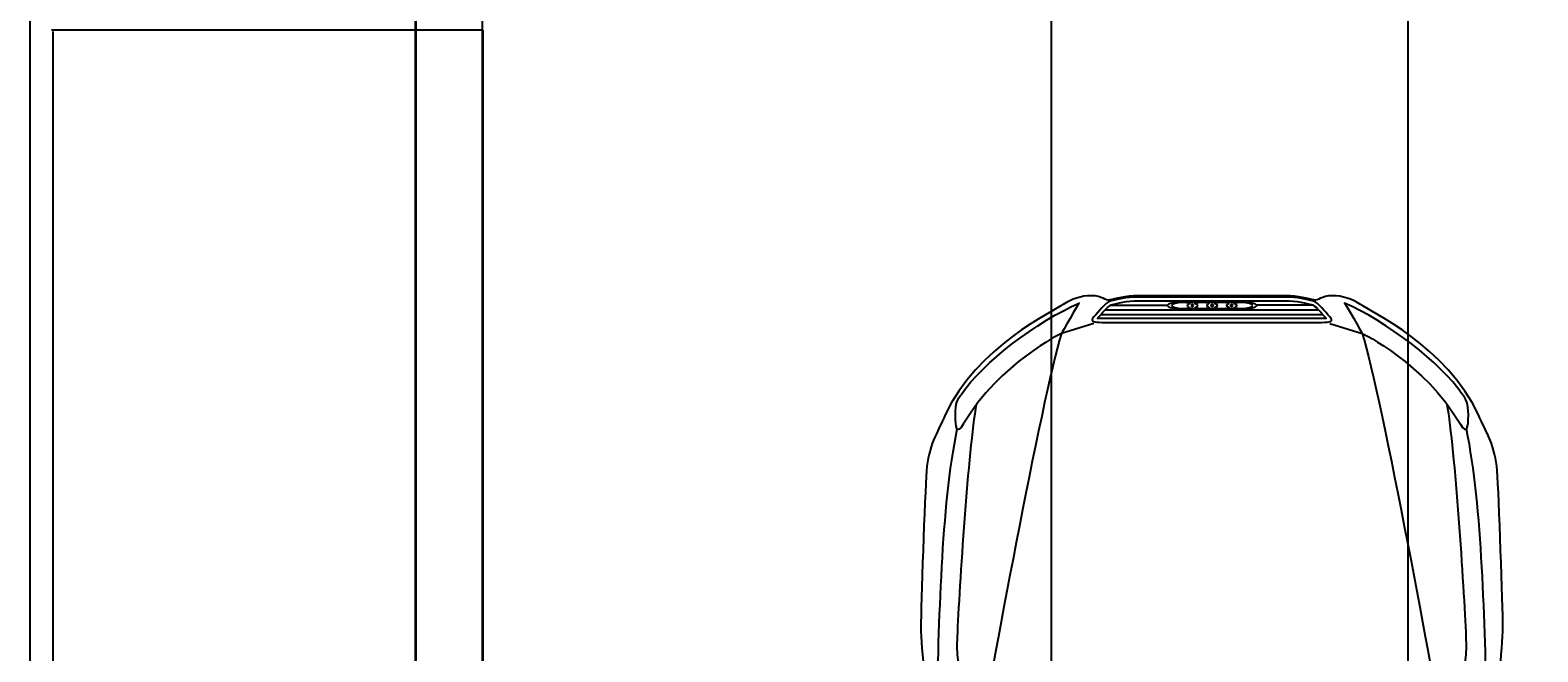
# Model space of a CAD drawing. Units: inches. Extents: x 2460 to 3031, y 933 to 2010.
# Tile 3 of 7: x 2460 to 2663, y 1256 to 1339. Entities that reach past the tile are written whole.
import ezdxf

# ---------------------------------------------------------------- set-up
doc = ezdxf.new("R2010")
doc.units = ezdxf.units.IN
for name, color, linetype, lineweight in [('A-ANNO-DIMS', 2, 'Continuous', 18), ('A-ANNO-TTLB', 7, 'Continuous', 25), ('AUDI', 7, 'Continuous', 25), ('C-PROP', 7, 'Continuous', 35)]:
    doc.layers.add(name, color=color, linetype=linetype, lineweight=lineweight)
doc.styles.get("Standard").update_dxf_attribs({"font": 'arial.ttf'})
doc.dimstyles.get("Standard").update_dxf_attribs({"dimtxt": 0.18, "dimasz": 0.18, "dimexe": 0.18, "dimexo": 0.0625, "dimgap": 0.09, "dimtad": 0, "dimtih": 1, "dimtoh": 1, "dimdec": 4, "dimzin": 0, "dimdsep": 46, "dimtxsty": 'Standard', "dimcen": 0.09, "dimadec": 0, "dimazin": 0, "dimtfac": 1, "dimtdec": 4, "dimtofl": 0, "dimtmove": 0, "dimatfit": 3, "dimfxl": 1, "dimtolj": 1, "dimtzin": 0, "dimarcsym": 0})

# ---------------------------------------------------------------- blocks, each defined once
blk = doc.blocks.new('*D35')
at = {"layer": 'A-ANNO-DIMS', "color": 0, "lineweight": -2, "transparency": 16777216}
for p, q in [((2520.61, 1339.48), (2462.69, 1339.48)), ((2462.87, 1339.3), (2462.87, 1197.91)), ((2462.87, 1056.16), (2462.87, 1197.55)), ((2511.61, 1055.98), (2462.69, 1055.98))]:
    blk.add_line(p, q, dxfattribs=at)
at = {"layer": 'A-ANNO-DIMS', "color": 0, "transparency": 16777216}
for points in [[(2462.84, 1339.3), (2462.9, 1339.3), (2462.87, 1339.48)], [(2462.84, 1056.16), (2462.9, 1056.16), (2462.87, 1055.98)]]:
    blk.add_solid(points, dxfattribs=at)
at = {"layer": 'Defpoints', "color": 0, "transparency": 16777216}
for p in [(2462.87, 1339.48), (2520.67, 1339.48), (2511.67, 1055.98)]:
    blk.add_point(p, dxfattribs=at)
at = {"layer": 'A-ANNO-DIMS', "color": 0, "transparency": 16777216, "insert": (2462.87, 1197.73), "char_height": 0.18, "attachment_point": 5}
blk.add_mtext('\\A1;283.5', dxfattribs=at)
blk = doc.blocks.new('*D37')
at = {"layer": 'A-ANNO-DIMS', "color": 0, "lineweight": -2, "transparency": 16777216}
for p, q in [((2597.17, 1554.98), (2597.17, 933.16)), ((2645.17, 1554.98), (2645.17, 933.16)), ((2597.35, 933.34), (2620.95, 933.34)), ((2644.99, 933.34), (2621.39, 933.34))]:
    blk.add_line(p, q, dxfattribs=at)
at = {"layer": 'A-ANNO-DIMS', "color": 0, "transparency": 16777216}
for points in [[(2597.35, 933.37), (2597.35, 933.31), (2597.17, 933.34)], [(2644.99, 933.37), (2644.99, 933.31), (2645.17, 933.34)]]:
    blk.add_solid(points, dxfattribs=at)
at = {"layer": 'Defpoints', "color": 0, "transparency": 16777216}
for p in [(2597.17, 1555.05), (2645.17, 1555.05), (2645.17, 933.34)]:
    blk.add_point(p, dxfattribs=at)
at = {"layer": 'A-ANNO-DIMS', "color": 0, "transparency": 16777216, "insert": (2621.17, 933.34), "char_height": 0.18, "attachment_point": 5}
blk.add_mtext('\\A1;48', dxfattribs=at)
blk = doc.blocks.new('*D40')
at = {"layer": 'A-ANNO-DIMS', "color": 0, "lineweight": -2, "transparency": 16777216}
for p, q in [((2511.67, 1056.05), (2511.67, 2006.96)), ((2511.85, 2006.78), (2516.02, 2006.78)), ((2520.49, 2006.78), (2516.32, 2006.78)), ((2520.67, 1056.05), (2520.67, 2006.96))]:
    blk.add_line(p, q, dxfattribs=at)
at = {"layer": 'A-ANNO-DIMS', "color": 0, "transparency": 16777216}
for points in [[(2511.85, 2006.81), (2511.85, 2006.75), (2511.67, 2006.78)], [(2520.49, 2006.81), (2520.49, 2006.75), (2520.67, 2006.78)]]:
    blk.add_solid(points, dxfattribs=at)
at = {"layer": 'Defpoints', "color": 0, "transparency": 16777216}
for p in [(2520.67, 2006.78), (2511.67, 1055.98), (2520.67, 1055.98)]:
    blk.add_point(p, dxfattribs=at)
at = {"layer": 'A-ANNO-DIMS', "color": 0, "transparency": 16777216, "insert": (2516.17, 2006.78), "char_height": 0.18, "attachment_point": 5}
blk.add_mtext('\\A1;9', dxfattribs=at)

msp = doc.modelspace()

# ---------------------------------------------------------------- linework, layer by layer
at = {"layer": 'A-ANNO-TTLB'}
msp.add_lwpolyline([(2459.8083, 2009.7942), (3030.6598, 2009.7942), (3030.6598, 936.3732), (2459.8083, 936.3732)], close=True, dxfattribs=at)
at = {"layer": 'AUDI'}
for points, knots in [([(2618.7829, 1107.9984), (2590.0793, 1108.312), (2585.9116, 1117.9641), (2584.1504, 1124.3238), (2584.1504, 1124.3238), (2583.0016, 1128.0786), (2582.0829, 1131.0667), (2581.6233, 1132.5994), (2581.6233, 1132.5994), (2581.1637, 1134.1318), (2580.1686, 1138.8059), (2580.0917, 1142.7138), (2580.0917, 1142.7138), (2580.0148, 1146.6218), (2579.6356, 1169.9218), (2579.6356, 1176.3523), (2579.6356, 1176.3523), (2579.6356, 1182.7825), (2579.6356, 1212.908), (2579.6356, 1217.1935), (2579.6356, 1217.1935), (2579.6356, 1221.4788), (2580.5514, 1238.5719), (2580.5514, 1244.012), (2580.5514, 1244.012), (2580.5514, 1249.4525), (2579.6356, 1256.2783), (2579.6356, 1259.1067), (2579.6356, 1259.1067), (2579.6356, 1261.9354), (2580.1681, 1276.8837), (2580.3981, 1280.1787), (2580.3981, 1280.1787), (2580.6281, 1283.4737), (2581.862, 1285.3424), (2582.9257, 1287.6881), (2582.9257, 1287.6881), (2587.0611, 1296.8058), (2597.6292, 1301.7862), (2598.7781, 1302.5527), (2598.7781, 1302.5527), (2599.9268, 1303.3191), (2601.1463, 1303.7354), (2602.6072, 1303.7354), (2602.6072, 1303.7354), (2604.0679, 1303.7354), (2604.4451, 1303.0127), (2605.0579, 1303.1658), (2605.0579, 1303.1658), (2605.6706, 1303.3191), (2607.1971, 1303.7354), (2608.8874, 1303.7354), (2608.8874, 1303.7354), (2610.5778, 1303.7354), (2618.7829, 1303.7354), (2618.7829, 1303.7354), (2618.7829, 1303.7354), (2618.7829, 1303.7354), (2626.988, 1303.7354), (2628.6784, 1303.7354), (2628.6784, 1303.7354), (2630.3689, 1303.7354), (2631.8952, 1303.3191), (2632.508, 1303.1658), (2632.508, 1303.1658), (2633.1208, 1303.0127), (2633.4979, 1303.7354), (2634.9587, 1303.7354), (2634.9587, 1303.7354), (2636.4196, 1303.7354), (2637.6391, 1303.3191), (2638.7878, 1302.5527), (2638.7878, 1302.5527), (2639.9365, 1301.7863), (2650.5047, 1296.8058), (2654.6402, 1287.6881), (2654.6402, 1287.6881), (2655.7038, 1285.3424), (2656.9377, 1283.4736), (2657.1677, 1280.1787), (2657.1677, 1280.1787), (2657.3978, 1276.8839), (2657.9302, 1261.9353), (2657.9302, 1259.1067), (2657.9302, 1259.1067), (2657.9302, 1256.2784), (2657.0145, 1249.4525), (2657.0145, 1244.012), (2657.0145, 1244.012), (2657.0145, 1238.5719), (2657.9302, 1221.4787), (2657.9302, 1217.1935), (2657.9302, 1217.1935), (2657.9302, 1212.908), (2657.9302, 1182.7824), (2657.9302, 1176.3523), (2657.9302, 1176.3523), (2657.9302, 1169.9218), (2657.5509, 1146.6216), (2657.4742, 1142.7138), (2657.4742, 1142.7138), (2657.3974, 1138.8059), (2656.4022, 1134.1318), (2655.9426, 1132.5994), (2655.9426, 1132.5994), (2655.4829, 1131.0667), (2654.5642, 1128.0785), (2653.4155, 1124.3238), (2653.4155, 1124.3238), (2651.6543, 1117.9641), (2647.4866, 1108.312), (2618.7829, 1107.9984)], [0, 0, 0, 0, 0.03571429, 0.03571429, 0.03571429, 0.0357143, 0.07142857, 0.07142857, 0.07142857, 0.07142858, 0.10714286, 0.10714286, 0.10714286, 0.10714287, 0.14285714, 0.14285714, 0.14285714, 0.14285715, 0.17857143, 0.17857143, 0.17857143, 0.17857144, 0.21428571, 0.21428571, 0.21428571, 0.21428572, 0.25, 0.25, 0.25, 0.25000001, 0.28571429, 0.28571429, 0.28571429, 0.2857143, 0.32142857, 0.32142857, 0.32142857, 0.32142858, 0.35714286, 0.35714286, 0.35714286, 0.35714287, 0.39285714, 0.39285714, 0.39285714, 0.39285715, 0.42857143, 0.42857143, 0.42857143, 0.42857144, 0.46428571, 0.46428571, 0.46428571, 0.46428572, 0.5, 0.5, 0.5, 0.50000001, 0.53571429, 0.53571429, 0.53571429, 0.5357143, 0.57142857, 0.57142857, 0.57142857, 0.57142858, 0.60714286, 0.60714286, 0.60714286, 0.60714287, 0.64285714, 0.64285714, 0.64285714, 0.64285715, 0.67857143, 0.67857143, 0.67857143, 0.67857144, 0.71428571, 0.71428571, 0.71428571, 0.71428572, 0.75, 0.75, 0.75, 0.75000001, 0.78571429, 0.78571429, 0.78571429, 0.7857143, 0.82142857, 0.82142857, 0.82142857, 0.82142858, 0.85714286, 0.85714286, 0.85714286, 0.85714287, 0.89285714, 0.89285714, 0.89285714, 0.89285715, 0.92857143, 0.92857143, 0.92857143, 0.92857144, 0.96428571, 0.96428571, 0.96428571, 0.96428572, 1, 1, 1, 1]), ([(2584.2757, 1287.7068), (2584.2757, 1286.0025), (2584.4712, 1284.9684), (2585.345, 1286.448), (2585.345, 1286.448), (2590.2526, 1294.7575), (2598.5576, 1298.6598), (2598.5576, 1298.6598), (2598.5576, 1298.6598), (2598.5576, 1298.6599), (2600.8077, 1302.6954), (2600.9485, 1302.7517), (2600.9485, 1302.7517), (2595.4691, 1300.4325), (2587.7735, 1294.5885), (2585.1565, 1290.5399), (2585.1565, 1290.5399), (2584.5274, 1289.7215), (2584.2757, 1289.3134), (2584.2757, 1287.7068)], [0, 0, 0, 0, 0.2, 0.2, 0.2, 0.20000001, 0.4, 0.4, 0.4, 0.40000001, 0.6, 0.6, 0.6, 0.60000001, 0.8, 0.8, 0.8, 0.80000001, 1, 1, 1, 1]), ([(2584.2757, 1287.7068), (2584.2757, 1286.0025), (2584.4712, 1284.9684), (2585.345, 1286.448), (2585.345, 1286.448), (2590.2526, 1294.7575), (2598.5576, 1298.6598), (2598.5576, 1298.6598), (2598.5576, 1298.6598), (2598.5576, 1298.6598), (2600.8077, 1302.6954), (2600.9485, 1302.7517), (2600.9485, 1302.7517), (2595.4691, 1300.4325), (2587.7735, 1294.5885), (2585.1565, 1290.5399), (2585.1565, 1290.5399), (2584.5274, 1289.7215), (2584.2757, 1289.3134), (2584.2757, 1287.7068)], [0, 0, 0, 0, 0.2, 0.2, 0.2, 0.20000001, 0.4, 0.4, 0.4, 0.40000001, 0.6, 0.6, 0.6, 0.60000001, 0.8, 0.8, 0.8, 0.80000001, 1, 1, 1, 1]), ([(2618.944, 1303.568), (2618.944, 1303.568), (2628.6784, 1303.568), (2628.6784, 1303.568), (2628.6784, 1303.568), (2630.2397, 1303.568), (2631.6569, 1303.2087), (2632.3377, 1303.0362), (2632.3377, 1303.0362), (2632.3377, 1303.0362), (2632.4673, 1303.0036), (2632.4673, 1303.0036), (2632.4673, 1303.0036), (2633.0863, 1302.8059), (2634.0439, 1301.5602), (2634.6506, 1300.8893), (2634.6506, 1300.8893), (2635.2573, 1300.2185), (2634.6506, 1300.1548), (2633.5651, 1300.1548), (2633.5651, 1300.1548), (2632.4796, 1300.1548), (2618.7829, 1300.1548), (2618.7829, 1300.1548), (2618.7829, 1300.1548), (2618.7829, 1300.1548), (2605.0863, 1300.1548), (2604.0008, 1300.1548), (2604.0008, 1300.1548), (2602.9153, 1300.1548), (2602.3086, 1300.2185), (2602.9153, 1300.8893), (2602.9153, 1300.8893), (2603.5219, 1301.5602), (2604.4796, 1302.8058), (2605.0986, 1303.0036), (2605.0986, 1303.0036), (2605.0986, 1303.0036), (2605.228, 1303.0364), (2605.228, 1303.0364), (2605.228, 1303.0364), (2605.909, 1303.2087), (2607.3262, 1303.5678), (2608.8874, 1303.5678), (2608.8874, 1303.5678), (2608.8874, 1303.5678), (2618.6219, 1303.568), (2618.6219, 1303.568), (2618.6219, 1303.568), (2618.6219, 1303.568), (2618.944, 1303.568), (2618.944, 1303.568)], [0, 0, 0, 0, 0.07692308, 0.07692308, 0.07692308, 0.07692309, 0.15384615, 0.15384615, 0.15384615, 0.15384616, 0.23076923, 0.23076923, 0.23076923, 0.23076924, 0.30769231, 0.30769231, 0.30769231, 0.30769232, 0.38461538, 0.38461538, 0.38461538, 0.38461539, 0.46153846, 0.46153846, 0.46153846, 0.46153847, 0.53846154, 0.53846154, 0.53846154, 0.53846155, 0.61538462, 0.61538462, 0.61538462, 0.61538463, 0.69230769, 0.69230769, 0.69230769, 0.6923077, 0.76923077, 0.76923077, 0.76923077, 0.76923078, 0.84615385, 0.84615385, 0.84615385, 0.84615386, 0.92307692, 0.92307692, 0.92307692, 0.92307693, 1, 1, 1, 1]), ([(2604.0008, 1300.6619), (2604.0008, 1300.6619), (2604.0008, 1300.6619), (2604.0008, 1300.6619), (2604.0008, 1300.6619), (2604.0008, 1300.6619), (2633.5651, 1300.6619), (2633.5651, 1300.6619), (2633.5651, 1300.6619), (2633.8147, 1300.6619), (2634.0067, 1300.668), (2634.1626, 1300.6776), (2634.1626, 1300.6776), (2634.043, 1300.8147), (2633.8584, 1301.0259), (2633.8584, 1301.0259), (2633.8584, 1301.0259), (2633.4141, 1301.5424), (2632.6708, 1302.4052), (2632.3141, 1302.5195), (2632.3141, 1302.5195), (2632.3141, 1302.5195), (2632.2138, 1302.5444), (2632.2138, 1302.5444), (2632.2138, 1302.5444), (2631.5503, 1302.7125), (2630.1751, 1303.0611), (2628.6784, 1303.0611), (2628.6784, 1303.0611), (2628.6784, 1303.0611), (2608.8874, 1303.0612), (2608.8874, 1303.0612), (2608.8874, 1303.0612), (2607.3908, 1303.0612), (2606.0156, 1302.7124), (2605.3542, 1302.5453), (2605.3542, 1302.5453), (2605.3542, 1302.5453), (2605.2225, 1302.5116), (2605.2225, 1302.5116), (2605.2225, 1302.5116), (2604.896, 1302.407), (2604.1523, 1301.5423), (2603.7075, 1301.0259), (2603.7075, 1301.0259), (2603.7075, 1301.0259), (2603.5233, 1300.8147), (2603.4033, 1300.6776), (2603.4033, 1300.6776), (2603.5595, 1300.6681), (2603.7511, 1300.6619), (2604.0008, 1300.6619)], [0, 0, 0, 0, 0.07692308, 0.07692308, 0.07692308, 0.07692309, 0.15384615, 0.15384615, 0.15384615, 0.15384616, 0.23076923, 0.23076923, 0.23076923, 0.23076924, 0.30769231, 0.30769231, 0.30769231, 0.30769232, 0.38461538, 0.38461538, 0.38461538, 0.38461539, 0.46153846, 0.46153846, 0.46153846, 0.46153847, 0.53846154, 0.53846154, 0.53846154, 0.53846155, 0.61538462, 0.61538462, 0.61538462, 0.61538463, 0.69230769, 0.69230769, 0.69230769, 0.6923077, 0.76923077, 0.76923077, 0.76923077, 0.76923078, 0.84615385, 0.84615385, 0.84615385, 0.84615386, 0.92307692, 0.92307692, 0.92307692, 0.92307693, 1, 1, 1, 1]), ([(2614.8352, 1301.8964), (2615.3502, 1301.8964), (2615.8006, 1301.9482), (2616.1542, 1302.0355), (2616.1542, 1302.0355), (2616.5085, 1301.9482), (2616.9912, 1301.8963), (2617.5063, 1301.8963), (2617.5063, 1301.8963), (2618.0208, 1301.8964), (2618.4713, 1301.9482), (2618.8253, 1302.0268), (2618.8253, 1302.0268), (2619.1465, 1301.9482), (2619.6301, 1301.8963), (2620.1124, 1301.8963), (2620.1124, 1301.8963), (2620.6275, 1301.8964), (2621.1102, 1301.9482), (2621.4642, 1302.0355), (2621.4642, 1302.0355), (2621.8181, 1301.9482), (2622.2685, 1301.8963), (2622.7832, 1301.8963), (2622.7832, 1301.8963), (2623.8778, 1301.8964), (2624.7787, 1302.1306), (2624.7787, 1302.4252), (2624.7787, 1302.4252), (2624.7787, 1302.7111), (2623.8778, 1302.9547), (2622.7832, 1302.9547), (2622.7832, 1302.9547), (2622.2685, 1302.9548), (2621.8181, 1302.894), (2621.4642, 1302.8154), (2621.4642, 1302.8154), (2621.1102, 1302.8941), (2620.6275, 1302.9547), (2620.1124, 1302.9547), (2620.1124, 1302.9547), (2619.6301, 1302.9548), (2619.1465, 1302.9027), (2618.8253, 1302.8154), (2618.8253, 1302.8154), (2618.4713, 1302.9028), (2618.0208, 1302.9547), (2617.5063, 1302.9547), (2617.5063, 1302.9547), (2616.9328, 1302.9548), (2616.3121, 1302.8508), (2616.1542, 1302.8154), (2616.1542, 1302.8154), (2615.8006, 1302.8941), (2615.3502, 1302.9547), (2614.8352, 1302.9547), (2614.8352, 1302.9547), (2613.7409, 1302.9548), (2612.8397, 1302.711), (2612.8397, 1302.4252), (2612.8397, 1302.4252), (2612.8397, 1302.1306), (2613.7409, 1301.8963), (2614.8352, 1301.8964)], [0, 0, 0, 0, 0.0625, 0.0625, 0.0625, 0.06250001, 0.125, 0.125, 0.125, 0.12500001, 0.1875, 0.1875, 0.1875, 0.18750001, 0.25, 0.25, 0.25, 0.25000001, 0.3125, 0.3125, 0.3125, 0.31250001, 0.375, 0.375, 0.375, 0.37500001, 0.4375, 0.4375, 0.4375, 0.43750001, 0.5, 0.5, 0.5, 0.50000001, 0.5625, 0.5625, 0.5625, 0.56250001, 0.625, 0.625, 0.625, 0.62500001, 0.6875, 0.6875, 0.6875, 0.68750001, 0.75, 0.75, 0.75, 0.75000001, 0.8125, 0.8125, 0.8125, 0.81250001, 0.875, 0.875, 0.875, 0.87500001, 0.9375, 0.9375, 0.9375, 0.93750001, 1, 1, 1, 1]), ([(2614.8352, 1301.8964), (2615.3502, 1301.8964), (2615.8006, 1301.9482), (2616.1542, 1302.0355), (2616.1542, 1302.0355), (2616.5085, 1301.9482), (2616.9912, 1301.8963), (2617.5063, 1301.8963), (2617.5063, 1301.8963), (2618.0208, 1301.8963), (2618.4713, 1301.9482), (2618.8253, 1302.0268), (2618.8253, 1302.0268), (2619.1465, 1301.9482), (2619.6301, 1301.8963), (2620.1124, 1301.8963), (2620.1124, 1301.8963), (2620.6275, 1301.8963), (2621.1102, 1301.9482), (2621.4642, 1302.0355), (2621.4642, 1302.0355), (2621.8181, 1301.9482), (2622.2685, 1301.8963), (2622.7832, 1301.8963), (2622.7832, 1301.8963), (2623.8778, 1301.8963), (2624.7787, 1302.1306), (2624.7787, 1302.4252), (2624.7787, 1302.4252), (2624.7787, 1302.7111), (2623.8778, 1302.9547), (2622.7832, 1302.9547), (2622.7832, 1302.9547), (2622.2685, 1302.9547), (2621.8181, 1302.894), (2621.4642, 1302.8154), (2621.4642, 1302.8154), (2621.1102, 1302.8941), (2620.6275, 1302.9547), (2620.1124, 1302.9547), (2620.1124, 1302.9547), (2619.6301, 1302.9547), (2619.1465, 1302.9027), (2618.8253, 1302.8154), (2618.8253, 1302.8154), (2618.4713, 1302.9028), (2618.0208, 1302.9547), (2617.5063, 1302.9547), (2617.5063, 1302.9547), (2616.9328, 1302.9547), (2616.3121, 1302.8508), (2616.1542, 1302.8154), (2616.1542, 1302.8154), (2615.8006, 1302.8941), (2615.3502, 1302.9547), (2614.8352, 1302.9547), (2614.8352, 1302.9547), (2613.7409, 1302.9547), (2612.8397, 1302.711), (2612.8397, 1302.4252), (2612.8397, 1302.4252), (2612.8397, 1302.1306), (2613.7409, 1301.8964), (2614.8352, 1301.8964)], [0, 0, 0, 0, 0.0625, 0.0625, 0.0625, 0.06250001, 0.125, 0.125, 0.125, 0.12500001, 0.1875, 0.1875, 0.1875, 0.18750001, 0.25, 0.25, 0.25, 0.25000001, 0.3125, 0.3125, 0.3125, 0.31250001, 0.375, 0.375, 0.375, 0.37500001, 0.4375, 0.4375, 0.4375, 0.43750001, 0.5, 0.5, 0.5, 0.50000001, 0.5625, 0.5625, 0.5625, 0.56250001, 0.625, 0.625, 0.625, 0.62500001, 0.6875, 0.6875, 0.6875, 0.68750001, 0.75, 0.75, 0.75, 0.75000001, 0.8125, 0.8125, 0.8125, 0.81250001, 0.875, 0.875, 0.875, 0.87500001, 0.9375, 0.9375, 0.9375, 0.93750001, 1, 1, 1, 1]), ([(2614.8352, 1302.8154), (2615.221, 1302.8154), (2615.5754, 1302.781), (2615.8329, 1302.711), (2615.8329, 1302.711), (2615.6395, 1302.6247), (2615.5107, 1302.5295), (2615.5107, 1302.4252), (2615.5107, 1302.4252), (2615.5107, 1302.3127), (2615.6395, 1302.2174), (2615.8329, 1302.1306), (2615.8329, 1302.1306), (2615.5754, 1302.07), (2615.221, 1302.0268), (2614.8352, 1302.0268), (2614.8352, 1302.0268), (2613.9984, 1302.0268), (2613.3547, 1302.2), (2613.3547, 1302.4252), (2613.3547, 1302.4252), (2613.3547, 1302.6421), (2613.9984, 1302.8154), (2614.8352, 1302.8154)], [0, 0, 0, 0, 0.16666667, 0.16666667, 0.16666667, 0.16666668, 0.33333333, 0.33333333, 0.33333333, 0.33333334, 0.5, 0.5, 0.5, 0.50000001, 0.66666667, 0.66666667, 0.66666667, 0.66666668, 0.83333333, 0.83333333, 0.83333333, 0.83333334, 1, 1, 1, 1]), ([(2616.3156, 1302.4253), (2616.3156, 1302.3559), (2616.2511, 1302.3038), (2616.1542, 1302.2519), (2616.1542, 1302.2519), (2616.0581, 1302.304), (2616.0258, 1302.3558), (2616.0258, 1302.4252), (2616.0258, 1302.4252), (2616.0258, 1302.4864), (2616.0581, 1302.5466), (2616.1542, 1302.5989), (2616.1542, 1302.5989), (2616.2511, 1302.5466), (2616.3156, 1302.4863), (2616.3156, 1302.4253)], [0, 0, 0, 0, 0.25, 0.25, 0.25, 0.25000001, 0.5, 0.5, 0.5, 0.50000001, 0.75, 0.75, 0.75, 0.75000001, 1, 1, 1, 1]), ([(2618.4713, 1302.7199), (2618.2779, 1302.6335), (2618.1497, 1302.5295), (2618.1497, 1302.4252), (2618.1497, 1302.4252), (2618.1497, 1302.3127), (2618.2779, 1302.2087), (2618.4713, 1302.1219), (2618.4713, 1302.1219), (2618.2143, 1302.0612), (2617.8921, 1302.0268), (2617.5063, 1302.0268), (2617.5063, 1302.0268), (2617.1195, 1302.0268), (2616.7661, 1302.07), (2616.5085, 1302.1306), (2616.5085, 1302.1306), (2616.7015, 1302.2176), (2616.8302, 1302.3126), (2616.8302, 1302.4252), (2616.8302, 1302.4252), (2616.8302, 1302.5296), (2616.7015, 1302.6247), (2616.5085, 1302.711), (2616.5085, 1302.711), (2616.7661, 1302.7811), (2617.1195, 1302.8154), (2617.5063, 1302.8154), (2617.5063, 1302.8154), (2617.8921, 1302.8154), (2618.2143, 1302.781), (2618.4713, 1302.7199)], [0, 0, 0, 0, 0.125, 0.125, 0.125, 0.12500001, 0.25, 0.25, 0.25, 0.25000001, 0.375, 0.375, 0.375, 0.37500001, 0.5, 0.5, 0.5, 0.50000001, 0.625, 0.625, 0.625, 0.62500001, 0.75, 0.75, 0.75, 0.75000001, 0.875, 0.875, 0.875, 0.87500001, 1, 1, 1, 1]), ([(2618.9858, 1302.4253), (2618.9858, 1302.3559), (2618.9221, 1302.2951), (2618.8253, 1302.2344), (2618.8253, 1302.2344), (2618.6965, 1302.2952), (2618.6324, 1302.3558), (2618.6324, 1302.4252), (2618.6324, 1302.4252), (2618.6324, 1302.4864), (2618.6965, 1302.5553), (2618.8253, 1302.6076), (2618.8253, 1302.6076), (2618.9221, 1302.5554), (2618.9858, 1302.4863), (2618.9858, 1302.4253)], [0, 0, 0, 0, 0.25, 0.25, 0.25, 0.25000001, 0.5, 0.5, 0.5, 0.50000001, 0.75, 0.75, 0.75, 0.75000001, 1, 1, 1, 1]), ([(2621.142, 1302.7111), (2620.9167, 1302.6247), (2620.7885, 1302.5295), (2620.7885, 1302.4252), (2620.7885, 1302.4252), (2620.7885, 1302.3127), (2620.9167, 1302.2174), (2621.142, 1302.1306), (2621.142, 1302.1306), (2620.8526, 1302.07), (2620.4987, 1302.0268), (2620.1124, 1302.0268), (2620.1124, 1302.0268), (2619.7584, 1302.0268), (2619.4044, 1302.0612), (2619.1465, 1302.1219), (2619.1465, 1302.1219), (2619.3726, 1302.2088), (2619.501, 1302.3126), (2619.501, 1302.4252), (2619.501, 1302.4252), (2619.501, 1302.5296), (2619.3726, 1302.6334), (2619.1465, 1302.7198), (2619.1465, 1302.7198), (2619.4044, 1302.7811), (2619.7584, 1302.8154), (2620.1124, 1302.8154), (2620.1124, 1302.8154), (2620.4987, 1302.8154), (2620.8526, 1302.781), (2621.142, 1302.7111)], [0, 0, 0, 0, 0.125, 0.125, 0.125, 0.12500001, 0.25, 0.25, 0.25, 0.25000001, 0.375, 0.375, 0.375, 0.37500001, 0.5, 0.5, 0.5, 0.50000001, 0.625, 0.625, 0.625, 0.62500001, 0.75, 0.75, 0.75, 0.75000001, 0.875, 0.875, 0.875, 0.87500001, 1, 1, 1, 1]), ([(2621.6247, 1302.4253), (2621.6247, 1302.3559), (2621.5606, 1302.3038), (2621.4642, 1302.2519), (2621.4642, 1302.2519), (2621.3673, 1302.304), (2621.303, 1302.3558), (2621.303, 1302.4252), (2621.303, 1302.4252), (2621.303, 1302.4864), (2621.3673, 1302.5466), (2621.4642, 1302.5989), (2621.4642, 1302.5989), (2621.5606, 1302.5466), (2621.6247, 1302.4863), (2621.6247, 1302.4253)], [0, 0, 0, 0, 0.25, 0.25, 0.25, 0.25000001, 0.5, 0.5, 0.5, 0.50000001, 0.75, 0.75, 0.75, 0.75000001, 1, 1, 1, 1]), ([(2624.2635, 1302.4253), (2624.2635, 1302.2001), (2623.6203, 1302.0268), (2622.7832, 1302.0268), (2622.7832, 1302.0268), (2622.3973, 1302.0268), (2622.0433, 1302.07), (2621.7858, 1302.1306), (2621.7858, 1302.1306), (2621.9792, 1302.2176), (2622.1075, 1302.3126), (2622.1075, 1302.4252), (2622.1075, 1302.4252), (2622.1075, 1302.5296), (2621.9792, 1302.6247), (2621.7858, 1302.711), (2621.7858, 1302.711), (2622.0433, 1302.7811), (2622.3973, 1302.8154), (2622.7832, 1302.8154), (2622.7832, 1302.8154), (2623.6203, 1302.8154), (2624.2635, 1302.6421), (2624.2635, 1302.4253)], [0, 0, 0, 0, 0.16666667, 0.16666667, 0.16666667, 0.16666668, 0.33333333, 0.33333333, 0.33333333, 0.33333334, 0.5, 0.5, 0.5, 0.50000001, 0.66666667, 0.66666667, 0.66666667, 0.66666668, 0.83333333, 0.83333333, 0.83333333, 0.83333334, 1, 1, 1, 1]), ([(2653.2902, 1287.7068), (2653.2902, 1286.0025), (2653.0947, 1284.9684), (2652.2209, 1286.448), (2652.2209, 1286.448), (2647.3133, 1294.7575), (2639.0083, 1298.6598), (2639.0083, 1298.6598), (2639.0083, 1298.6598), (2639.0083, 1298.6599), (2636.7582, 1302.6954), (2636.6172, 1302.7517), (2636.6172, 1302.7517), (2642.0966, 1300.4325), (2649.7923, 1294.5885), (2652.4094, 1290.5399), (2652.4094, 1290.5399), (2653.0383, 1289.7215), (2653.2902, 1289.3134), (2653.2902, 1287.7068)], [0, 0, 0, 0, 0.2, 0.2, 0.2, 0.20000001, 0.4, 0.4, 0.4, 0.40000001, 0.6, 0.6, 0.6, 0.60000001, 0.8, 0.8, 0.8, 0.80000001, 1, 1, 1, 1]), ([(2653.2902, 1287.7068), (2653.2902, 1286.0025), (2653.0947, 1284.9684), (2652.2209, 1286.448), (2652.2209, 1286.448), (2647.3133, 1294.7575), (2639.0083, 1298.6598), (2639.0083, 1298.6598), (2639.0083, 1298.6598), (2639.0083, 1298.6598), (2636.7582, 1302.6954), (2636.6172, 1302.7517), (2636.6172, 1302.7517), (2642.0966, 1300.4325), (2649.7923, 1294.5885), (2652.4094, 1290.5399), (2652.4094, 1290.5399), (2653.0383, 1289.7215), (2653.2902, 1289.3134), (2653.2902, 1287.7068)], [0, 0, 0, 0, 0.2, 0.2, 0.2, 0.20000001, 0.4, 0.4, 0.4, 0.40000001, 0.6, 0.6, 0.6, 0.60000001, 0.8, 0.8, 0.8, 0.80000001, 1, 1, 1, 1]), ([(2587.9301, 1245.7186), (2587.0363, 1247.5072), (2584.263, 1251.0766), (2584.5585, 1257.8216), (2584.5585, 1257.8216), (2584.8541, 1264.5669), (2586.0517, 1283.1771), (2587.1263, 1289.0978)], [0, 0, 0, 0, 0.5, 0.5, 0.5, 0.50000001, 1, 1, 1, 1]), ([(2649.6356, 1245.7186), (2650.5296, 1247.5072), (2653.3028, 1251.0766), (2653.0074, 1257.8216), (2653.0074, 1257.8216), (2652.7118, 1264.5669), (2651.5142, 1283.1771), (2650.4396, 1289.0978)], [0, 0, 0, 0, 0.5, 0.5, 0.5, 0.50000001, 1, 1, 1, 1]), ([(2585.4965, 1124.2398), (2584.0544, 1131.455), (2582.5189, 1146.0668), (2582.2566, 1161.2842), (2582.2566, 1161.2842), (2581.9943, 1176.5015), (2581.3391, 1235.0091), (2581.7324, 1247.34), (2581.7324, 1247.34), (2582.1256, 1259.6711), (2582.3457, 1275.227), (2584.5301, 1285.8147)], [0, 0, 0, 0, 0.33333333, 0.33333333, 0.33333333, 0.33333334, 0.66666667, 0.66666667, 0.66666667, 0.66666668, 1, 1, 1, 1]), ([(2652.0694, 1124.2398), (2653.5115, 1131.455), (2655.047, 1146.0668), (2655.3092, 1161.2842), (2655.3092, 1161.2842), (2655.5716, 1176.5015), (2656.2267, 1235.0091), (2655.8335, 1247.34), (2655.8335, 1247.34), (2655.4402, 1259.6711), (2655.2202, 1275.227), (2653.0358, 1285.8147)], [0, 0, 0, 0, 0.33333333, 0.33333333, 0.33333333, 0.33333334, 0.66666667, 0.66666667, 0.66666667, 0.66666668, 1, 1, 1, 1])]:
    msp.add_open_spline(points, degree=3, knots=knots, dxfattribs=at)
for points in [[(2605.0981, 1302.4475), (2605.0981, 1302.4475), (2612.8397, 1302.4475), (2612.8397, 1302.4475)], [(2632.4678, 1302.4475), (2632.4678, 1302.4475), (2624.7262, 1302.4475), (2624.7262, 1302.4475)], [(2603.8716, 1301.2163), (2603.8716, 1301.2163), (2633.6594, 1301.2163), (2633.6594, 1301.2163)], [(2604.4364, 1301.8452), (2604.4364, 1301.8452), (2633.0465, 1301.8452), (2633.0465, 1301.8452)], [(2598.5576, 1298.6599), (2596.0301, 1290.615), (2588.3637, 1249.4001), (2587.9167, 1245.3755)], [(2602.9052, 1299.9959), (2602.9052, 1299.9959), (2598.5576, 1298.6599), (2598.5576, 1298.6599)], [(2634.6606, 1299.9959), (2634.6606, 1299.9959), (2639.0083, 1298.6599), (2639.0083, 1298.6599)], [(2639.0083, 1298.6599), (2641.5358, 1290.615), (2649.2022, 1249.4001), (2649.6492, 1245.3755)]]:
    msp.add_open_spline(points, degree=3, dxfattribs=at)
at = {"layer": 'C-PROP'}
for p, q in [((2511.6684, 1957.9828), (2511.6684, 1055.9828)), ((2511.6684, 1957.9828), (2511.6684, 1055.9828)), ((2520.6684, 1339.4828), (2520.6684, 1055.9828))]:
    msp.add_line(p, q, dxfattribs=at)

# ---------------------------------------------------------------- dimensions: what is measured, and where the dimension line sits
at = {"layer": 'A-ANNO-DIMS'}
for base, p1, p2, picture, middle in [((2520.6684, 2006.7823), (2511.6684, 1055.9828), (2520.6684, 1055.9828), '*D40', (2516.1684, 2006.7823)), ((2645.1684, 933.3411), (2597.1684, 1555.0454), (2645.1684, 1555.0454), '*D37', (2621.1684, 933.3411))]:
    dim = msp.add_linear_dim(base=base, p1=p1, p2=p2, dimstyle='Standard', override={"dimdec": 0, "dimlfac": 1, "dimrnd": 0, "dimzin": 0, "dimdsep": 46, "dimlunit": 2}, dxfattribs=at)
    dim.commit()
    dim.dimension.update_dxf_attribs({"geometry": picture, "text_midpoint": middle})
dim = msp.add_linear_dim(base=(2462.8689, 1339.4828), p1=(2511.6684, 1055.9828), p2=(2520.6684, 1339.4828), angle=90, dimstyle='Standard', override={"dimdec": 1, "dimlfac": 1, "dimrnd": 0, "dimzin": 0, "dimdsep": 46, "dimlunit": 2}, dxfattribs=at)
dim.commit()
dim.dimension.update_dxf_attribs({"geometry": '*D35', "text_midpoint": (2462.8689, 1197.7328)})

doc.saveas('drawing.dxf')
